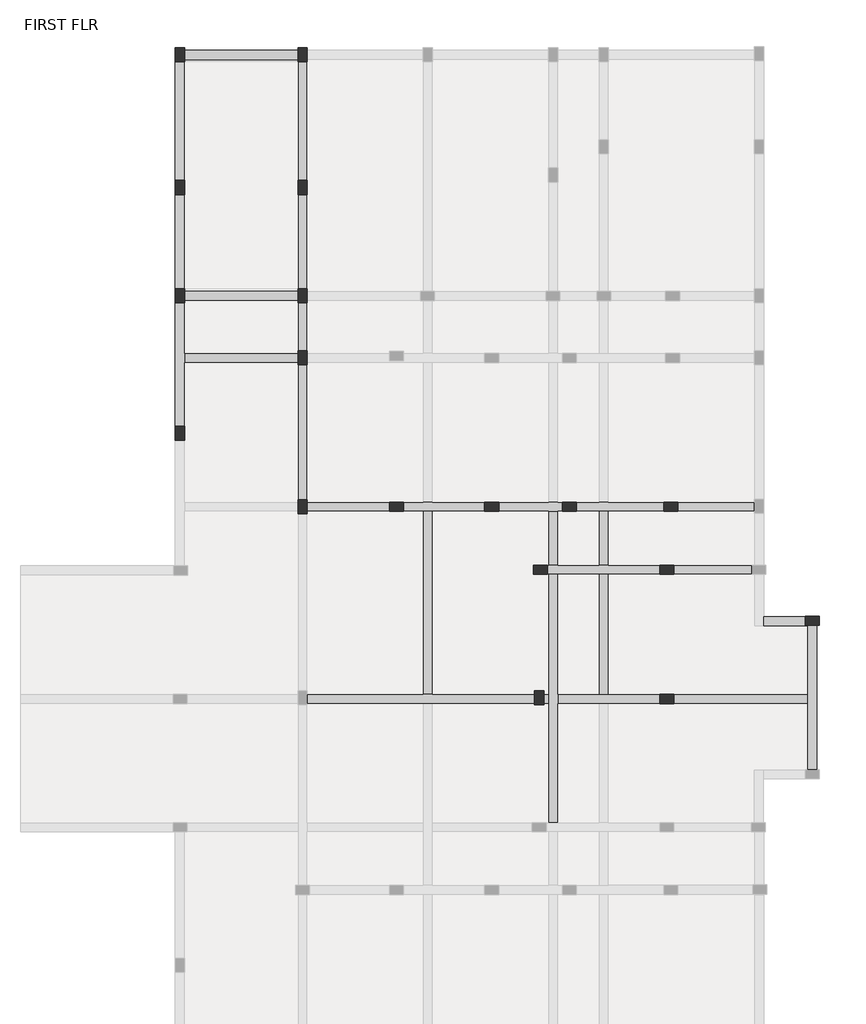
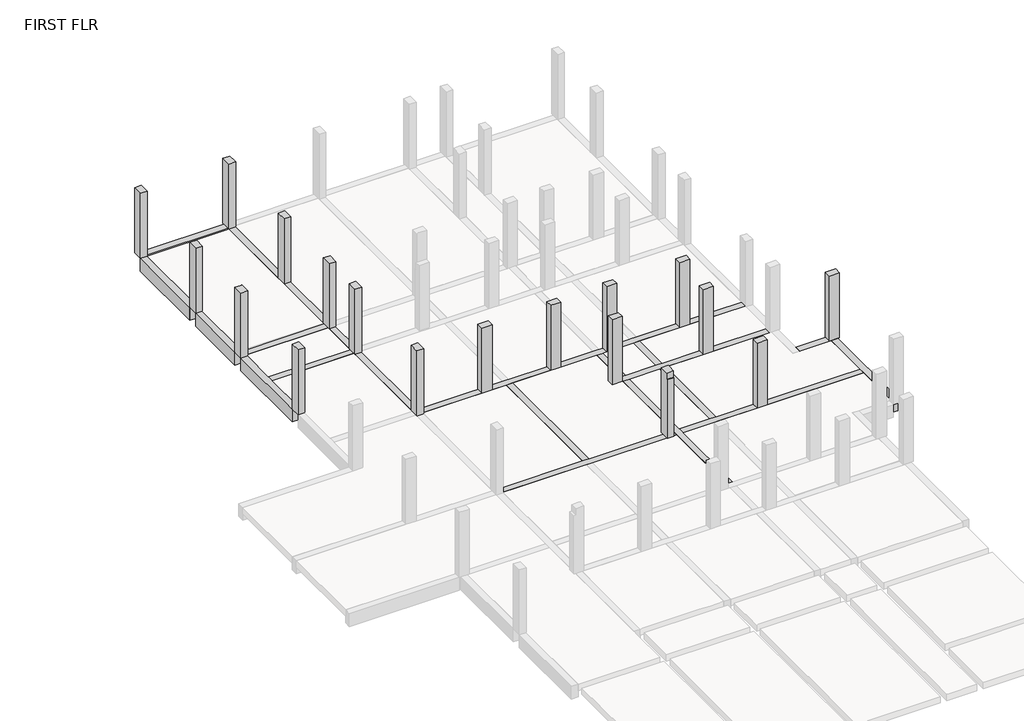
# One storey, part 4 of 5: 28 beams, 18 columns.
"""IFC4 building model written with IfcOpenShell, lengths in millimetres."""

from ifc_helpers import new_model, si_unit, frame, origin, place, context, project, spatial, polyline, outline, extrude, faceted_brep, element, save

model = new_model("IFC4")

# Units and contexts
model_context = context("Model", 3, world=origin())
ifc_project = project(units=[si_unit("LENGTHUNIT", "METRE", prefix="MILLI")], contexts=[model_context])

# Site, building, storey
site = spatial("IfcSite", under=ifc_project)
building = spatial("IfcBuilding", under=site)
storey = spatial("IfcBuildingStorey", under=building, Name="FIRST FLR", Elevation=3000.0)

# Beams
placement = place(None, origin())
element("IfcBeam", 1, ObjectType="M_Concrete-Rectangular Beam : 300 x 600mm", at=placement, inside=storey, context=model_context, shape_type="SweptSolid", body=[
    extrude(outline(polyline([(-1971.7865686, 21837.8349362), (-1971.7865686, 21537.8349362), (-5591.7865686, 21537.8349362), (-5591.7865686, 21837.8349362), (-1971.7865686, 21837.8349362)])), frame((0.0, 0.0, 2400.0), z_axis=(0.0, 0.0, 1.0), x_axis=(1.0, 0.0, 0.0)), (0.0, 0.0, 1.0), 600.0),
])
element("IfcBeam", 2, ObjectType="M_Concrete-Rectangular Beam : 300 x 600mm", at=placement, inside=storey, context=model_context, shape_type="Brep", body=[
    faceted_brep([(-5891.7865686, 21462.8349362, 3000.0), (-5891.7865686, 17662.8349362, 3000.0), (-5888.8105653, 17662.8349362, 3000.0), (-5888.8105653, 17674.7148651, 3000.0), (-5591.7865686, 17674.7148651, 3000.0), (-5591.7865686, 21462.8349362, 3000.0), (-5891.7865686, 21462.8349362, 2400.0), (-5891.7865686, 17662.8349362, 2400.0), (-5591.7865686, 21462.8349362, 2400.0), (-5591.7865686, 17674.7148651, 2400.0), (-5888.8105653, 17674.7148651, 2400.0), (-5888.8105653, 17662.8349362, 2400.0), (-5591.7865686, 17674.7148651, 2700.0), (-5591.7865686, 21462.8349362, 2700.0)], [[[0, 1, 2, 3, 4, 5]], [[1, 0, 6, 7]], [[7, 6, 8, 9, 10, 11]], [[5, 4, 12, 9, 8, 13]], [[8, 6, 0, 5, 13]], [[1, 7, 11, 2]], [[10, 3, 2, 11]], [[3, 10, 9, 12, 4]]]),
])
element("IfcBeam", 3, ObjectType="M_Concrete-Rectangular Beam : 300 x 600mm", at=placement, inside=storey, context=model_context, shape_type="SweptSolid", body=[
    extrude(outline(polyline([(3000.0, -5888.8105653), (2400.0, -5888.8105653), (2400.0, -5588.8105653), (2700.0, -5588.8105653), (2700.0, -5591.7865686), (3000.0, -5591.7865686), (3000.0, -5888.8105653)])), frame((0.0, 14212.5179708, 0.0), z_axis=(0.0, 1.0, 0.0), x_axis=(0.0, 0.0, 1.0)), (0.0, 0.0, 1.0), 3012.1968944),
])
element("IfcBeam", 4, ObjectType="M_Concrete-Rectangular Beam : 300 x 600mm", at=placement, inside=storey, context=model_context, shape_type="Brep", body=[
    faceted_brep([(-5888.8105653, 13762.5179708, 3000.0), (-5888.8105653, 9817.5252033, 3000.0), (-5588.8105653, 9817.5252033, 3000.0), (-5588.8105653, 11857.4075451, 3000.0), (-5588.8105653, 12157.4075451, 3000.0), (-5588.8105653, 13762.5179708, 3000.0), (-5888.8105653, 13762.5179708, 2400.0), (-5888.8105653, 9817.5252033, 2400.0), (-5588.8105653, 13762.5179708, 2400.0), (-5588.8105653, 12157.4075451, 2400.0), (-5588.8105653, 11857.4075451, 2400.0), (-5588.8105653, 9817.5252033, 2400.0), (-5588.8105653, 13762.5179708, 2700.0), (-5588.8105653, 9817.5252033, 2700.0)], [[[0, 1, 2, 3, 4, 5]], [[1, 0, 6, 7]], [[7, 6, 8, 9, 10, 11]], [[11, 10, 9, 8, 12, 5, 4, 3, 2, 13]], [[8, 6, 0, 5, 12]], [[2, 1, 7, 11, 13]]]),
])
element("IfcBeam", 5, ObjectType="M_Concrete-Rectangular Beam : 300 x 600mm", at=placement, inside=storey, context=model_context, shape_type="Brep", body=[
    faceted_brep([(14319.1163908, 3443.0536525, 3000.0), (14619.1163908, 3443.0536525, 3000.0), (14619.1163908, 3443.0536525, 2400.0), (14319.1163908, 3443.0536525, 2400.0), (14319.1163908, 3435.7536525, 3000.0), (14319.1163908, 1251.1713929, 3000.0), (14319.1163908, 951.1713929, 3000.0), (14319.1163908, -1148.8286071, 3000.0), (14619.1163908, -1148.8286071, 3000.0), (14619.1163908, -1148.8286071, 2400.0), (14319.1163908, -1148.8286071, 2400.0), (14319.1163908, 951.1713929, 2400.0), (14319.1163908, 1251.1713929, 2400.0), (14319.1163908, 3435.7536525, 2400.0), (14319.1163908, -1148.8286071, 2700.0)], [[[0, 1, 2, 3]], [[1, 0, 4, 5, 6, 7, 8]], [[2, 1, 8, 9]], [[3, 2, 9, 10, 11, 12, 13]], [[0, 3, 13, 12, 11, 10, 14, 7, 6, 5, 4]], [[7, 14, 10, 9, 8]]]),
])
element("IfcBeam", 6, ObjectType="M_Concrete-Rectangular Beam : 300 x 600mm", at=placement, inside=storey, context=model_context, shape_type="Brep", body=[
    faceted_brep([(12916.8679014, 3735.7536525, 3000.0), (12916.8679014, 3435.7536525, 3000.0), (14319.1163908, 3435.7536525, 3000.0), (14319.1163908, 3443.0536525, 3000.0), (14619.1163908, 3443.0536525, 3000.0), (14619.1163908, 3455.7536525, 3000.0), (14244.1163908, 3455.7536525, 3000.0), (14244.1163908, 3735.7536525, 3000.0), (12916.8679014, 3735.7536525, 2400.0), (14244.1163908, 3735.7536525, 2400.0), (12916.8679014, 3435.7536525, 2400.0), (14244.1163908, 3455.7536525, 2400.0), (14619.1163908, 3455.7536525, 2400.0), (14619.1163908, 3443.0536525, 2400.0), (14319.1163908, 3443.0536525, 2400.0), (14319.1163908, 3435.7536525, 2400.0), (12916.8679014, 3435.7536525, 2700.0), (14319.1163908, 3435.7536525, 2700.0)], [[[0, 1, 2, 3, 4, 5, 6, 7]], [[8, 0, 7, 9]], [[10, 8, 9, 11, 12, 13, 14, 15]], [[2, 1, 16, 10, 15, 17]], [[1, 0, 8, 10, 16]], [[12, 5, 4, 13]], [[7, 6, 11, 9]], [[11, 6, 5, 12]], [[3, 14, 13, 4]], [[14, 3, 2, 17, 15]]]),
])
element("IfcBeam", 7, ObjectType="M_Concrete-Rectangular Beam : 300 x 600mm", at=placement, inside=storey, context=model_context, shape_type="Brep", body=[
    faceted_brep([(-1671.7865686, 21462.8349362, 3000.0), (-1971.7865686, 21462.8349362, 3000.0), (-1971.7865686, 17674.7148651, 3000.0), (-1671.7865686, 17674.7148651, 3000.0), (-1971.7865686, 21462.8349362, 2700.0), (-1971.7865686, 21462.8349362, 2400.0), (-1971.7865686, 17674.7148651, 2400.0), (-1971.7865686, 17674.7148651, 2700.0), (-1671.7865686, 21462.8349362, 2400.0), (-1671.7865686, 17674.7148651, 2400.0), (-1671.7865686, 17674.7148651, 2700.0), (-1671.7865686, 21462.8349362, 2700.0)], [[[0, 1, 2, 3]], [[2, 1, 4, 5, 6, 7]], [[5, 8, 9, 6]], [[0, 3, 10, 9, 8, 11]], [[1, 0, 11, 8, 5, 4]], [[3, 2, 7, 6, 9, 10]]]),
])
element("IfcBeam", 8, ObjectType="M_Concrete-Rectangular Beam : 300 x 600mm", at=placement, inside=storey, context=model_context, shape_type="Brep", body=[
    faceted_brep([(-1671.7865686, 17224.7148651, 3000.0), (-1971.7865686, 17224.7148651, 3000.0), (-1971.7865686, 14212.5179708, 3000.0), (-1671.7865686, 14212.5179708, 3000.0), (-1971.7865686, 17224.7148651, 2700.0), (-1971.7865686, 17224.7148651, 2400.0), (-1971.7865686, 14212.5179708, 2400.0), (-1971.7865686, 14212.5179708, 2700.0), (-1671.7865686, 17224.7148651, 2400.0), (-1671.7865686, 14212.5179708, 2400.0), (-1671.7865686, 14212.5179708, 2700.0), (-1671.7865686, 17224.7148651, 2700.0)], [[[0, 1, 2, 3]], [[2, 1, 4, 5, 6, 7]], [[5, 8, 9, 6]], [[0, 3, 10, 9, 8, 11]], [[1, 0, 11, 8, 5, 4]], [[3, 2, 7, 6, 9, 10]]]),
])
element("IfcBeam", 9, ObjectType="M_Concrete-Rectangular Beam : 300 x 600mm", at=placement, inside=storey, context=model_context, shape_type="Brep", body=[
    faceted_brep([(-1671.7865686, 13762.5179708, 3000.0), (-1971.7865686, 13762.5179708, 3000.0), (-1971.7865686, 12232.4075451, 3000.0), (-1671.7865686, 12232.4075451, 3000.0), (-1971.7865686, 13762.5179708, 2700.0), (-1971.7865686, 13762.5179708, 2400.0), (-1971.7865686, 12232.4075451, 2400.0), (-1971.7865686, 12232.4075451, 2700.0), (-1671.7865686, 13762.5179708, 2400.0), (-1671.7865686, 12232.4075451, 2400.0), (-1671.7865686, 12232.4075451, 2700.0), (-1671.7865686, 13762.5179708, 2700.0)], [[[0, 1, 2, 3]], [[2, 1, 4, 5, 6, 7]], [[5, 8, 9, 6]], [[0, 3, 10, 9, 8, 11]], [[1, 0, 11, 8, 5, 4]], [[3, 2, 7, 6, 9, 10]]]),
])
element("IfcBeam", 10, ObjectType="M_Concrete-Rectangular Beam : 300 x 600mm", at=placement, inside=storey, context=model_context, shape_type="Brep", body=[
    faceted_brep([(-1671.7865686, 11782.4075451, 3000.0), (-1971.7865686, 11782.4075451, 3000.0), (-1971.7865686, 7474.7076276, 3000.0), (-1671.7865686, 7474.7076276, 3000.0), (-1971.7865686, 11782.4075451, 2700.0), (-1971.7865686, 11782.4075451, 2400.0), (-1971.7865686, 7474.7076276, 2400.0), (-1971.7865686, 7474.7076276, 2700.0), (-1671.7865686, 11782.4075451, 2400.0), (-1671.7865686, 7474.7076276, 2400.0), (-1671.7865686, 7474.7076276, 2700.0), (-1671.7865686, 11782.4075451, 2700.0)], [[[0, 1, 2, 3]], [[2, 1, 4, 5, 6, 7]], [[5, 8, 9, 6]], [[0, 3, 10, 9, 8, 11]], [[1, 0, 11, 8, 5, 4]], [[3, 2, 7, 6, 9, 10]]]),
])
element("IfcBeam", 11, ObjectType="M_Concrete-Rectangular Beam : 300 x 600mm", at=placement, inside=storey, context=model_context, shape_type="Brep", body=[
    faceted_brep([(-5588.8105653, 14137.5179708, 3000.0), (-5588.8105653, 13837.5179708, 3000.0), (-1971.7865686, 13837.5179708, 3000.0), (-1971.7865686, 14137.5179708, 3000.0), (-5588.8105653, 13837.5179708, 2700.0), (-5588.8105653, 13837.5179708, 2400.0), (-1971.7865686, 13837.5179708, 2400.0), (-1971.7865686, 13837.5179708, 2700.0), (-5588.8105653, 14137.5179708, 2400.0), (-1971.7865686, 14137.5179708, 2400.0)], [[[0, 1, 2, 3]], [[2, 1, 4, 5, 6, 7]], [[5, 8, 9, 6]], [[8, 0, 3, 9]], [[1, 0, 8, 5, 4]], [[9, 3, 2, 7, 6]]]),
])
element("IfcBeam", 12, ObjectType="M_Concrete-Rectangular Beam : 300 x 600mm", at=placement, inside=storey, context=model_context, shape_type="Brep", body=[
    faceted_brep([(-1971.7865686, 11857.4075451, 3000.0), (-1971.7865686, 12157.4075451, 3000.0), (-5588.8105653, 12157.4075451, 3000.0), (-5588.8105653, 11857.4075451, 3000.0), (-5588.8105653, 11857.4075451, 2700.0), (-5588.8105653, 11857.4075451, 2400.0), (-1971.7865686, 11857.4075451, 2400.0), (-1971.7865686, 11857.4075451, 2700.0), (-1971.7865686, 12157.4075451, 2400.0), (-5588.8105653, 12157.4075451, 2400.0), (-1971.7865686, 12157.4075451, 2700.0), (-5588.8105653, 12157.4075451, 2700.0)], [[[0, 1, 2, 3]], [[0, 3, 4, 5, 6, 7]], [[8, 6, 5, 9]], [[2, 1, 10, 8, 9, 11]], [[1, 0, 7, 6, 8, 10]], [[3, 2, 11, 9, 5, 4]]]),
])
element("IfcBeam", 13, ObjectType="M_Concrete-Rectangular Beam : 300 x 600mm", at=placement, inside=storey, context=model_context, shape_type="Brep", body=[
    faceted_brep([(-1671.7865686, 7399.7076276, 3000.0), (-1671.7865686, 7099.7076276, 3000.0), (949.7296816, 7099.7076276, 3000.0), (949.7296816, 7399.7076276, 3000.0), (-1671.7865686, 7099.7076276, 2700.0), (-1671.7865686, 7099.7076276, 2400.0), (949.7296816, 7099.7076276, 2400.0), (949.7296816, 7099.7076276, 2700.0), (-1671.7865686, 7399.7076276, 2400.0), (949.7296816, 7399.7076276, 2400.0), (949.7296816, 7399.7076276, 2700.0), (-1671.7865686, 7399.7076276, 2700.0)], [[[0, 1, 2, 3]], [[2, 1, 4, 5, 6, 7]], [[5, 8, 9, 6]], [[0, 3, 10, 9, 8, 11]], [[1, 0, 11, 8, 5, 4]], [[3, 2, 7, 6, 9, 10]]]),
])
element("IfcBeam", 14, ObjectType="M_Concrete-Rectangular Beam : 300 x 600mm", at=placement, inside=storey, context=model_context, shape_type="Brep", body=[
    faceted_brep([(1399.7296816, 7399.7076276, 3000.0), (1399.7296816, 7099.7076276, 3000.0), (2024.7296816, 7099.7076276, 3000.0), (2324.7296816, 7099.7076276, 3000.0), (3997.5248054, 7099.7076276, 3000.0), (3997.5248054, 7399.7076276, 3000.0), (2324.7296816, 7399.7076276, 3000.0), (2024.7296816, 7399.7076276, 3000.0), (1399.7296816, 7099.7076276, 2400.0), (2024.7296816, 7099.7076276, 2400.0), (2324.7296816, 7099.7076276, 2400.0), (3997.5248054, 7099.7076276, 2400.0), (3997.5248054, 7099.7076276, 2700.0), (1399.7296816, 7099.7076276, 2700.0), (1399.7296816, 7399.7076276, 2400.0), (2024.7296816, 7399.7076276, 2400.0), (2324.7296816, 7399.7076276, 2400.0), (3997.5248054, 7399.7076276, 2400.0), (1399.7296816, 7399.7076276, 2700.0), (3997.5248054, 7399.7076276, 2700.0)], [[[0, 1, 2, 3, 4, 5, 6, 7]], [[8, 9, 10, 11, 12, 4, 3, 2, 1, 13]], [[8, 14, 15, 16, 17, 11, 10, 9]], [[17, 16, 15, 14, 18, 0, 7, 6, 5, 19]], [[1, 0, 18, 14, 8, 13]], [[5, 4, 12, 11, 17, 19]]]),
])
element("IfcBeam", 15, ObjectType="M_Concrete-Rectangular Beam : 300 x 600mm", at=placement, inside=storey, context=model_context, shape_type="Brep", body=[
    faceted_brep([(4447.5248054, 7399.7076276, 3000.0), (4447.5248054, 7099.7076276, 3000.0), (6032.5248054, 7099.7076276, 3000.0), (6332.5248054, 7099.7076276, 3000.0), (6481.8679014, 7099.7076276, 3000.0), (6481.8679014, 7399.7076276, 3000.0), (6332.5248054, 7399.7076276, 3000.0), (6032.5248054, 7399.7076276, 3000.0), (4447.5248054, 7099.7076276, 2400.0), (6032.5248054, 7099.7076276, 2400.0), (6332.5248054, 7099.7076276, 2400.0), (6481.8679014, 7099.7076276, 2400.0), (6481.8679014, 7099.7076276, 2700.0), (4447.5248054, 7099.7076276, 2700.0), (4447.5248054, 7399.7076276, 2400.0), (6032.5248054, 7399.7076276, 2400.0), (6332.5248054, 7399.7076276, 2400.0), (6481.8679014, 7399.7076276, 2400.0), (4447.5248054, 7399.7076276, 2700.0), (6481.8679014, 7399.7076276, 2700.0)], [[[0, 1, 2, 3, 4, 5, 6, 7]], [[8, 9, 10, 11, 12, 4, 3, 2, 1, 13]], [[8, 14, 15, 16, 17, 11, 10, 9]], [[17, 16, 15, 14, 18, 0, 7, 6, 5, 19]], [[1, 0, 18, 14, 8, 13]], [[5, 4, 12, 11, 17, 19]]]),
])
element("IfcBeam", 16, ObjectType="M_Concrete-Rectangular Beam : 300 x 600mm", at=placement, inside=storey, context=model_context, shape_type="Brep", body=[
    faceted_brep([(6931.8679014, 7399.7076276, 3000.0), (6931.8679014, 7099.7076276, 3000.0), (7656.8679014, 7099.7076276, 3000.0), (7956.8679014, 7099.7076276, 3000.0), (9721.8679014, 7099.7076276, 3000.0), (9721.8679014, 7399.7076276, 3000.0), (7956.8679014, 7399.7076276, 3000.0), (7656.8679014, 7399.7076276, 3000.0), (6931.8679014, 7099.7076276, 2400.0), (7656.8679014, 7099.7076276, 2400.0), (7956.8679014, 7099.7076276, 2400.0), (9721.8679014, 7099.7076276, 2400.0), (9721.8679014, 7099.7076276, 2700.0), (6931.8679014, 7099.7076276, 2700.0), (6931.8679014, 7399.7076276, 2400.0), (7656.8679014, 7399.7076276, 2400.0), (7956.8679014, 7399.7076276, 2400.0), (9721.8679014, 7399.7076276, 2400.0), (6931.8679014, 7399.7076276, 2700.0), (9721.8679014, 7399.7076276, 2700.0)], [[[0, 1, 2, 3, 4, 5, 6, 7]], [[8, 9, 10, 11, 12, 4, 3, 2, 1, 13]], [[8, 14, 15, 16, 17, 11, 10, 9]], [[17, 16, 15, 14, 18, 0, 7, 6, 5, 19]], [[1, 0, 18, 14, 8, 13]], [[5, 4, 12, 11, 17, 19]]]),
])
element("IfcBeam", 17, ObjectType="M_Concrete-Rectangular Beam : 300 x 600mm", at=placement, inside=storey, context=model_context, shape_type="Brep", body=[
    faceted_brep([(6007.5248054, 5387.6057249, 3000.0), (6007.5248054, 5087.6057249, 3000.0), (6032.5248054, 5087.6057249, 3000.0), (6332.5248054, 5087.6057249, 3000.0), (7656.8679014, 5087.6057249, 3000.0), (7956.8679014, 5087.6057249, 3000.0), (9601.8679014, 5087.6057249, 3000.0), (9601.8679014, 5387.6057249, 3000.0), (7956.8679014, 5387.6057249, 3000.0), (7656.8679014, 5387.6057249, 3000.0), (6332.5248054, 5387.6057249, 3000.0), (6032.5248054, 5387.6057249, 3000.0), (6007.5248054, 5087.6057249, 2400.0), (6032.5248054, 5087.6057249, 2400.0), (6332.5248054, 5087.6057249, 2400.0), (7656.8679014, 5087.6057249, 2400.0), (7956.8679014, 5087.6057249, 2400.0), (9601.8679014, 5087.6057249, 2400.0), (9601.8679014, 5087.6057249, 2700.0), (6007.5248054, 5087.6057249, 2700.0), (6007.5248054, 5387.6057249, 2400.0), (6032.5248054, 5387.6057249, 2400.0), (6332.5248054, 5387.6057249, 2400.0), (7656.8679014, 5387.6057249, 2400.0), (7956.8679014, 5387.6057249, 2400.0), (9601.8679014, 5387.6057249, 2400.0), (6007.5248054, 5387.6057249, 2700.0), (9601.8679014, 5387.6057249, 2700.0)], [[[0, 1, 2, 3, 4, 5, 6, 7, 8, 9, 10, 11]], [[12, 13, 14, 15, 16, 17, 18, 6, 5, 4, 3, 2, 1, 19]], [[12, 20, 21, 22, 23, 24, 25, 17, 16, 15, 14, 13]], [[25, 24, 23, 22, 21, 20, 26, 0, 11, 10, 9, 8, 7, 27]], [[1, 0, 26, 20, 12, 19]], [[7, 6, 18, 17, 25, 27]]]),
])
element("IfcBeam", 18, ObjectType="M_Concrete-Rectangular Beam : 300 x 600mm", at=placement, inside=storey, context=model_context, shape_type="Brep", body=[
    faceted_brep([(10051.8679014, 5387.6057249, 3000.0), (10051.8679014, 5087.6057249, 3000.0), (12541.8679014, 5087.6057249, 3000.0), (12541.8679014, 5387.6057249, 3000.0), (10051.8679014, 5087.6057249, 2700.0), (10051.8679014, 5087.6057249, 2400.0), (12541.8679014, 5087.6057249, 2400.0), (12541.8679014, 5087.6057249, 2700.0), (10051.8679014, 5387.6057249, 2400.0), (12541.8679014, 5387.6057249, 2400.0), (12541.8679014, 5387.6057249, 2700.0), (10051.8679014, 5387.6057249, 2700.0)], [[[0, 1, 2, 3]], [[2, 1, 4, 5, 6, 7]], [[5, 8, 9, 6]], [[0, 3, 10, 9, 8, 11]], [[1, 0, 11, 8, 5, 4]], [[3, 2, 7, 6, 9, 10]]]),
])
element("IfcBeam", 19, ObjectType="M_Concrete-Rectangular Beam : 300 x 600mm", at=placement, inside=storey, context=model_context, shape_type="Brep", body=[
    faceted_brep([(10051.8679014, 1251.1713929, 3000.0), (10051.8679014, 951.1713929, 3000.0), (14319.1163908, 951.1713929, 3000.0), (14319.1163908, 1251.1713929, 3000.0), (10051.8679014, 951.1713929, 2700.0), (10051.8679014, 951.1713929, 2400.0), (14319.1163908, 951.1713929, 2400.0), (14319.1163908, 951.1713929, 2700.0), (10051.8679014, 1251.1713929, 2400.0), (14319.1163908, 1251.1713929, 2400.0), (14319.1163908, 1251.1713929, 2700.0), (10051.8679014, 1251.1713929, 2700.0)], [[[0, 1, 2, 3]], [[2, 1, 4, 5, 6, 7]], [[5, 8, 9, 6]], [[0, 3, 10, 9, 8, 11]], [[1, 0, 11, 8, 5, 4]], [[3, 2, 7, 6, 9, 10]]]),
])
element("IfcBeam", 20, ObjectType="M_Concrete-Rectangular Beam : 300 x 600mm", at=placement, inside=storey, context=model_context, shape_type="Brep", body=[
    faceted_brep([(6032.5248054, 951.1713929, 3000.0), (6032.5248054, 1251.1713929, 3000.0), (5892.5248054, 1251.1713929, 3000.0), (5892.5248054, 951.1713929, 3000.0), (5892.5248054, 951.1713929, 2700.0), (5892.5248054, 951.1713929, 2400.0), (6032.5248054, 951.1713929, 2400.0), (6032.5248054, 951.1713929, 2700.0), (6032.5248054, 1251.1713929, 2400.0), (5892.5248054, 1251.1713929, 2400.0), (6032.5248054, 1251.1713929, 2700.0), (5892.5248054, 1251.1713929, 2700.0)], [[[0, 1, 2, 3]], [[0, 3, 4, 5, 6, 7]], [[8, 6, 5, 9]], [[2, 1, 10, 8, 9, 11]], [[1, 0, 7, 6, 8, 10]], [[3, 2, 11, 9, 5, 4]]]),
    faceted_brep([(-1671.7865686, 951.1713929, 3000.0), (-1671.7865686, 1251.1713929, 3000.0), (-1671.7865686, 1251.1713929, 2700.0), (-1671.7865686, 1251.1713929, 2400.0), (-1671.7865686, 951.1713929, 2400.0), (-1671.7865686, 951.1713929, 2700.0), (5592.5248054, 1251.1713929, 3000.0), (5592.5248054, 951.1713929, 3000.0), (5592.5248054, 951.1713929, 2700.0), (5592.5248054, 951.1713929, 2400.0), (5592.5248054, 1251.1713929, 2400.0), (5592.5248054, 1251.1713929, 2700.0), (2024.7296816, 951.1713929, 3000.0), (2324.7296816, 951.1713929, 3000.0), (2324.7296816, 1251.1713929, 3000.0), (2024.7296816, 1251.1713929, 3000.0), (2024.7296816, 951.1713929, 2400.0), (2324.7296816, 951.1713929, 2400.0), (2024.7296816, 1251.1713929, 2400.0), (2324.7296816, 1251.1713929, 2400.0)], [[[0, 1, 2, 3, 4, 5]], [[6, 7, 8, 9, 10, 11]], [[1, 0, 12, 13, 7, 6, 14, 15]], [[4, 16, 17, 9, 8, 7, 13, 12, 0, 5]], [[4, 3, 18, 19, 10, 9, 17, 16]], [[10, 19, 18, 3, 2, 1, 15, 14, 6, 11]]]),
])
element("IfcBeam", 21, ObjectType="M_Concrete-Rectangular Beam : 300 x 600mm", at=placement, inside=storey, context=model_context, shape_type="Brep", body=[
    faceted_brep([(2324.7296816, 7099.7076276, 3000.0), (2024.7296816, 7099.7076276, 3000.0), (2024.7296816, 1251.1713929, 3000.0), (2324.7296816, 1251.1713929, 3000.0), (2024.7296816, 7099.7076276, 2700.0), (2024.7296816, 7099.7076276, 2400.0), (2024.7296816, 1251.1713929, 2400.0), (2024.7296816, 1251.1713929, 2700.0), (2324.7296816, 7099.7076276, 2400.0), (2324.7296816, 5387.6057249, 2400.0), (2324.7296816, 5087.6057249, 2400.0), (2324.7296816, 1251.1713929, 2400.0), (2324.7296816, 1251.1713929, 2700.0), (2324.7296816, 7099.7076276, 2700.0)], [[[0, 1, 2, 3]], [[2, 1, 4, 5, 6, 7]], [[5, 8, 9, 10, 11, 6]], [[0, 3, 12, 11, 10, 9, 8, 13]], [[1, 0, 13, 8, 5, 4]], [[3, 2, 7, 6, 11, 12]]]),
])
element("IfcBeam", 22, ObjectType="M_Concrete-Rectangular Beam : 300 x 600mm", at=placement, inside=storey, context=model_context, shape_type="Brep", body=[
    faceted_brep([(6332.5248054, 7099.7076276, 3000.0), (6032.5248054, 7099.7076276, 3000.0), (6032.5248054, 5387.6057249, 3000.0), (6332.5248054, 5387.6057249, 3000.0), (6032.5248054, 7099.7076276, 2700.0), (6032.5248054, 7099.7076276, 2400.0), (6032.5248054, 5387.6057249, 2400.0), (6032.5248054, 5387.6057249, 2700.0), (6332.5248054, 7099.7076276, 2400.0), (6332.5248054, 5387.6057249, 2400.0), (6332.5248054, 5387.6057249, 2700.0), (6332.5248054, 7099.7076276, 2700.0)], [[[0, 1, 2, 3]], [[2, 1, 4, 5, 6, 7]], [[5, 8, 9, 6]], [[0, 3, 10, 9, 8, 11]], [[1, 0, 11, 8, 5, 4]], [[3, 2, 7, 6, 9, 10]]]),
])
element("IfcBeam", 23, ObjectType="M_Concrete-Rectangular Beam : 300 x 600mm", at=placement, inside=storey, context=model_context, shape_type="Brep", body=[
    faceted_brep([(7956.8679014, 7099.7076276, 3000.0), (7656.8679014, 7099.7076276, 3000.0), (7656.8679014, 5387.6057249, 3000.0), (7956.8679014, 5387.6057249, 3000.0), (7656.8679014, 7099.7076276, 2700.0), (7656.8679014, 7099.7076276, 2400.0), (7656.8679014, 5387.6057249, 2400.0), (7656.8679014, 5387.6057249, 2700.0), (7956.8679014, 7099.7076276, 2400.0), (7956.8679014, 5387.6057249, 2400.0), (7956.8679014, 5387.6057249, 2700.0), (7956.8679014, 7099.7076276, 2700.0)], [[[0, 1, 2, 3]], [[2, 1, 4, 5, 6, 7]], [[5, 8, 9, 6]], [[0, 3, 10, 9, 8, 11]], [[1, 0, 11, 8, 5, 4]], [[3, 2, 7, 6, 9, 10]]]),
])
element("IfcBeam", 24, ObjectType="M_Concrete-Rectangular Beam : 300 x 600mm", at=placement, inside=storey, context=model_context, shape_type="Brep", body=[
    faceted_brep([(6332.5248054, 5087.6057249, 3000.0), (6032.5248054, 5087.6057249, 3000.0), (6032.5248054, 1251.1713929, 3000.0), (6032.5248054, 951.1713929, 3000.0), (6032.5248054, -2839.4535766, 3000.0), (6332.5248054, -2839.4535766, 3000.0), (6332.5248054, 951.1713929, 3000.0), (6332.5248054, 1251.1713929, 3000.0), (6032.5248054, 5087.6057249, 2400.0), (6032.5248054, 1251.1713929, 2400.0), (6032.5248054, 951.1713929, 2400.0), (6032.5248054, -2839.4535766, 2400.0), (6032.5248054, -2839.4535766, 2700.0), (6032.5248054, 5087.6057249, 2700.0), (6332.5248054, 5087.6057249, 2400.0), (6332.5248054, 1251.1713929, 2400.0), (6332.5248054, 951.1713929, 2400.0), (6332.5248054, -2839.4535766, 2400.0), (6332.5248054, 5087.6057249, 2700.0), (6332.5248054, -2839.4535766, 2700.0)], [[[0, 1, 2, 3, 4, 5, 6, 7]], [[8, 9, 10, 11, 12, 4, 3, 2, 1, 13]], [[8, 14, 15, 16, 17, 11, 10, 9]], [[17, 16, 15, 14, 18, 0, 7, 6, 5, 19]], [[1, 0, 18, 14, 8, 13]], [[5, 4, 12, 11, 17, 19]]]),
])
element("IfcBeam", 25, ObjectType="M_Concrete-Rectangular Beam : 300 x 600mm", at=placement, inside=storey, context=model_context, shape_type="Brep", body=[
    faceted_brep([(7956.8679014, 5087.6057249, 3000.0), (7656.8679014, 5087.6057249, 3000.0), (7656.8679014, 1251.1713929, 3000.0), (7956.8679014, 1251.1713929, 3000.0), (7656.8679014, 5087.6057249, 2700.0), (7656.8679014, 5087.6057249, 2400.0), (7656.8679014, 1251.1713929, 2400.0), (7656.8679014, 1251.1713929, 2700.0), (7956.8679014, 5087.6057249, 2400.0), (7956.8679014, 1251.1713929, 2400.0), (7956.8679014, 1251.1713929, 2700.0), (7956.8679014, 5087.6057249, 2700.0)], [[[0, 1, 2, 3]], [[2, 1, 4, 5, 6, 7]], [[5, 8, 9, 6]], [[0, 3, 10, 9, 8, 11]], [[1, 0, 11, 8, 5, 4]], [[3, 2, 7, 6, 9, 10]]]),
])
element("IfcBeam", 26, ObjectType="M_Concrete-Rectangular Beam : 300 x 600mm", at=placement, inside=storey, context=model_context, shape_type="Brep", body=[
    faceted_brep([(9601.8679014, 951.1713929, 3000.0), (9601.8679014, 1251.1713929, 3000.0), (7956.8679014, 1251.1713929, 3000.0), (7656.8679014, 1251.1713929, 3000.0), (6332.5248054, 1251.1713929, 3000.0), (6332.5248054, 951.1713929, 3000.0), (7656.8679014, 951.1713929, 3000.0), (7956.8679014, 951.1713929, 3000.0), (6332.5248054, 951.1713929, 2400.0), (7656.8679014, 951.1713929, 2400.0), (7956.8679014, 951.1713929, 2400.0), (9601.8679014, 951.1713929, 2400.0), (9601.8679014, 951.1713929, 2700.0), (6332.5248054, 951.1713929, 2700.0), (9601.8679014, 1251.1713929, 2400.0), (6332.5248054, 1251.1713929, 2400.0), (7656.8679014, 1251.1713929, 2400.0), (7956.8679014, 1251.1713929, 2400.0), (6332.5248054, 1251.1713929, 2700.0), (9601.8679014, 1251.1713929, 2700.0)], [[[0, 1, 2, 3, 4, 5, 6, 7]], [[8, 9, 10, 11, 12, 0, 7, 6, 5, 13]], [[14, 11, 10, 9, 8, 15, 16, 17]], [[14, 17, 16, 15, 18, 4, 3, 2, 1, 19]], [[1, 0, 12, 11, 14, 19]], [[5, 4, 18, 15, 8, 13]]]),
])
element("IfcBeam", 27, ObjectType="M_Concrete-Rectangular Beam : 300 x 600mm", at=placement, inside=storey, context=model_context, shape_type="Brep", body=[
    faceted_brep([(10171.8679014, 7399.7076276, 3000.0), (10171.8679014, 7099.7076276, 3000.0), (12616.8679014, 7099.7076276, 3000.0), (12616.8679014, 7399.7076276, 3000.0), (10171.8679014, 7099.7076276, 2700.0), (10171.8679014, 7099.7076276, 2400.0), (12616.8679014, 7099.7076276, 2400.0), (12616.8679014, 7099.7076276, 2700.0), (10171.8679014, 7399.7076276, 2400.0), (12616.8679014, 7399.7076276, 2400.0), (12616.8679014, 7399.7076276, 2700.0), (10171.8679014, 7399.7076276, 2700.0)], [[[0, 1, 2, 3]], [[2, 1, 4, 5, 6, 7]], [[5, 8, 9, 6]], [[0, 3, 10, 9, 8, 11]], [[8, 5, 4, 1, 0, 11]], [[3, 2, 7, 6, 9, 10]]]),
])
element("IfcBeam", 28, ObjectType="M_Concrete-Rectangular Beam : 300 x 600mm", at=placement, inside=storey, context=model_context, shape_type="SweptSolid", body=[
    extrude(outline(polyline([(5557.5248054, 5387.6057249), (5557.5248054, 5087.6057249), (2324.7296816, 5087.6057249), (2324.7296816, 5387.6057249), (5557.5248054, 5387.6057249)])), frame((0.0, 0.0, 2400.0), z_axis=(0.0, 0.0, 1.0), x_axis=(1.0, 0.0, 0.0)), (0.0, 0.0, 1.0), 300.0),
])

# Columns
element("IfcColumn", 29, ObjectType="M_Concrete-Rectangular-Column : 300 x 450mm", at=placement, inside=storey, context=model_context, shape_type="SweptSolid", body=[
    extrude(outline(polyline([(-5591.7865686, 21912.8349362), (-5591.7865686, 21462.8349362), (-5891.7865686, 21462.8349362), (-5891.7865686, 21912.8349362), (-5591.7865686, 21912.8349362)])), frame((0.0, 0.0, 3000.0), z_axis=(0.0, 0.0, 1.0), x_axis=(1.0, 0.0, 0.0)), (0.0, 0.0, 1.0), 3048.0),
])
element("IfcColumn", 30, ObjectType="M_Concrete-Rectangular-Column : 300 x 450mm", at=placement, inside=storey, context=model_context, shape_type="Brep", body=[
    faceted_brep([(-1671.7865686, 21912.8349362, 3000.0), (-1671.7865686, 21462.8349362, 3000.0), (-1971.7865686, 21462.8349362, 3000.0), (-1971.7865686, 21912.8349362, 3000.0), (-1671.7865686, 21912.8349362, 6048.0), (-1671.7865686, 21537.8349362, 6048.0), (-1671.7865686, 21462.8349362, 6048.0), (-1671.7865686, 21462.8349362, 5748.0), (-1971.7865686, 21462.8349362, 6048.0), (-1971.7865686, 21462.8349362, 5748.0), (-1971.7865686, 21912.8349362, 6048.0)], [[[0, 1, 2, 3]], [[1, 0, 4, 5, 6, 7]], [[2, 1, 7, 6, 8, 9]], [[3, 2, 9, 8, 10]], [[0, 3, 10, 4]], [[8, 6, 5, 4, 10]]]),
])
element("IfcColumn", 31, ObjectType="M_Concrete-Rectangular-Column : 300 x 450mm", at=placement, inside=storey, context=model_context, shape_type="Brep", body=[
    faceted_brep([(-1671.7865686, 17674.7148651, 3000.0), (-1671.7865686, 17224.7148651, 3000.0), (-1971.7865686, 17224.7148651, 3000.0), (-1971.7865686, 17674.7148651, 3000.0), (-1671.7865686, 17674.7148651, 5748.0), (-1671.7865686, 17674.7148651, 6048.0), (-1671.7865686, 17224.7148651, 6048.0), (-1671.7865686, 17224.7148651, 5748.0), (-1971.7865686, 17224.7148651, 6048.0), (-1971.7865686, 17224.7148651, 5748.0), (-1971.7865686, 17674.7148651, 6048.0), (-1971.7865686, 17674.7148651, 5748.0)], [[[0, 1, 2, 3]], [[1, 0, 4, 5, 6, 7]], [[2, 1, 7, 6, 8, 9]], [[3, 2, 9, 8, 10, 11]], [[0, 3, 11, 10, 5, 4]], [[6, 5, 10, 8]]]),
])
element("IfcColumn", 32, ObjectType="M_Concrete-Rectangular-Column : 300 x 450mm", at=placement, inside=storey, context=model_context, shape_type="SweptSolid", body=[
    extrude(outline(polyline([(3000.0, -5888.8105653), (3000.0, -5588.8105653), (5748.0, -5588.8105653), (5748.0, -5591.7865686), (6048.0, -5591.7865686), (6048.0, -5888.8105653), (3000.0, -5888.8105653)])), frame((0.0, 17224.7148651, 0.0), z_axis=(0.0, 1.0, 0.0), x_axis=(0.0, 0.0, 1.0)), (0.0, 0.0, 1.0), 450.0),
])
element("IfcColumn", 33, ObjectType="M_Concrete-Rectangular-Column : 300 x 450mm", at=placement, inside=storey, context=model_context, shape_type="Brep", body=[
    faceted_brep([(-5588.8105653, 14212.5179708, 3000.0), (-5588.8105653, 13762.5179708, 3000.0), (-5888.8105653, 13762.5179708, 3000.0), (-5888.8105653, 14212.5179708, 3000.0), (-5588.8105653, 14212.5179708, 5748.0), (-5588.8105653, 14212.5179708, 6048.0), (-5588.8105653, 13837.5179708, 6048.0), (-5588.8105653, 13762.5179708, 6048.0), (-5588.8105653, 13762.5179708, 5748.0), (-5888.8105653, 13762.5179708, 6048.0), (-5888.8105653, 14212.5179708, 6048.0), (-5591.7865686, 14212.5179708, 6048.0)], [[[0, 1, 2, 3]], [[1, 0, 4, 5, 6, 7, 8]], [[2, 1, 8, 7, 9]], [[3, 2, 9, 10]], [[0, 3, 10, 11, 5, 4]], [[9, 7, 6, 5, 11, 10]]]),
])
element("IfcColumn", 34, ObjectType="M_Concrete-Rectangular-Column : 300 x 450mm", at=placement, inside=storey, context=model_context, shape_type="Brep", body=[
    faceted_brep([(-1671.7865686, 14212.5179708, 3000.0), (-1671.7865686, 13762.5179708, 3000.0), (-1971.7865686, 13762.5179708, 3000.0), (-1971.7865686, 14212.5179708, 3000.0), (-1671.7865686, 14212.5179708, 5748.0), (-1671.7865686, 14212.5179708, 6048.0), (-1671.7865686, 14137.5179708, 6048.0), (-1671.7865686, 13837.5179708, 6048.0), (-1671.7865686, 13762.5179708, 6048.0), (-1671.7865686, 13762.5179708, 5748.0), (-1971.7865686, 13762.5179708, 6048.0), (-1971.7865686, 13762.5179708, 5748.0), (-1971.7865686, 13837.5179708, 6048.0), (-1971.7865686, 14212.5179708, 6048.0), (-1971.7865686, 14212.5179708, 5748.0)], [[[0, 1, 2, 3]], [[1, 0, 4, 5, 6, 7, 8, 9]], [[2, 1, 9, 8, 10, 11]], [[3, 2, 11, 10, 12, 13, 14]], [[0, 3, 14, 13, 5, 4]], [[10, 8, 7, 6, 5, 13, 12]]]),
])
element("IfcColumn", 35, ObjectType="M_Concrete-Rectangular-Column : 300 x 450mm", at=placement, inside=storey, context=model_context, shape_type="Brep", body=[
    faceted_brep([(-1971.7865686, 11782.4075451, 3000.0), (-1971.7865686, 12232.4075451, 3000.0), (-1671.7865686, 12232.4075451, 3000.0), (-1671.7865686, 11782.4075451, 3000.0), (-1971.7865686, 11782.4075451, 5748.0), (-1971.7865686, 11782.4075451, 6048.0), (-1971.7865686, 11857.4075451, 6048.0), (-1971.7865686, 12157.4075451, 6048.0), (-1971.7865686, 12232.4075451, 6048.0), (-1971.7865686, 12232.4075451, 5748.0), (-1671.7865686, 12232.4075451, 6048.0), (-1671.7865686, 12232.4075451, 5748.0), (-1671.7865686, 12157.4075451, 6048.0), (-1671.7865686, 11857.4075451, 6048.0), (-1671.7865686, 11782.4075451, 6048.0), (-1671.7865686, 11782.4075451, 5748.0)], [[[0, 1, 2, 3]], [[1, 0, 4, 5, 6, 7, 8, 9]], [[2, 1, 9, 8, 10, 11]], [[3, 2, 11, 10, 12, 13, 14, 15]], [[0, 3, 15, 14, 5, 4]], [[10, 8, 7, 6, 5, 14, 13, 12]]]),
])
element("IfcColumn", 36, ObjectType="M_Concrete-Rectangular-Column : 300 x 450mm", at=placement, inside=storey, context=model_context, shape_type="Brep", body=[
    faceted_brep([(-5888.8105653, 9367.5252033, 3000.0), (-5888.8105653, 9817.5252033, 3000.0), (-5588.8105653, 9817.5252033, 3000.0), (-5588.8105653, 9367.5252033, 3000.0), (-5888.8105653, 9367.5252033, 6048.0), (-5888.8105653, 9817.5252033, 6048.0), (-5588.8105653, 9817.5252033, 6048.0), (-5588.8105653, 9817.5252033, 5748.0), (-5588.8105653, 9367.5252033, 6048.0), (-5588.8105653, 9367.5252033, 5748.0)], [[[0, 1, 2, 3]], [[1, 0, 4, 5]], [[2, 1, 5, 6, 7]], [[3, 2, 7, 6, 8, 9]], [[0, 3, 9, 8, 4]], [[5, 4, 8, 6]]]),
])
element("IfcColumn", 37, ObjectType="M_Concrete-Rectangular-Column : 300 x 450mm", at=placement, inside=storey, context=model_context, shape_type="Brep", body=[
    faceted_brep([(-1971.7865686, 7024.7076276, 3000.0), (-1971.7865686, 7474.7076276, 3000.0), (-1671.7865686, 7474.7076276, 3000.0), (-1671.7865686, 7024.7076276, 3000.0), (-1971.7865686, 7024.7076276, 5748.0), (-1971.7865686, 7024.7076276, 6048.0), (-1971.7865686, 7099.7076276, 6048.0), (-1971.7865686, 7399.7076276, 6048.0), (-1971.7865686, 7474.7076276, 6048.0), (-1971.7865686, 7474.7076276, 5748.0), (-1671.7865686, 7474.7076276, 6048.0), (-1671.7865686, 7474.7076276, 5748.0), (-1671.7865686, 7399.7076276, 6048.0), (-1671.7865686, 7099.7076276, 6048.0), (-1671.7865686, 7024.7076276, 6048.0), (-1671.7865686, 7024.7076276, 5748.0)], [[[0, 1, 2, 3]], [[1, 0, 4, 5, 6, 7, 8, 9]], [[2, 1, 9, 8, 10, 11]], [[3, 2, 11, 10, 12, 13, 14, 15]], [[0, 3, 15, 14, 5, 4]], [[10, 8, 7, 6, 5, 14, 13, 12]]]),
])
element("IfcColumn", 38, ObjectType="M_Concrete-Rectangular-Column : 300 x 450mm", at=placement, inside=storey, context=model_context, shape_type="Brep", body=[
    faceted_brep([(1399.7296816, 7099.7076276, 3000.0), (949.7296816, 7099.7076276, 3000.0), (949.7296816, 7399.7076276, 3000.0), (1399.7296816, 7399.7076276, 3000.0), (1399.7296816, 7099.7076276, 5748.0), (1399.7296816, 7099.7076276, 6048.0), (949.7296816, 7099.7076276, 6048.0), (949.7296816, 7099.7076276, 5748.0), (949.7296816, 7399.7076276, 6048.0), (949.7296816, 7399.7076276, 5748.0), (1399.7296816, 7399.7076276, 6048.0), (1399.7296816, 7399.7076276, 5748.0)], [[[0, 1, 2, 3]], [[1, 0, 4, 5, 6, 7]], [[2, 1, 7, 6, 8, 9]], [[3, 2, 9, 8, 10, 11]], [[0, 3, 11, 10, 5, 4]], [[6, 5, 10, 8]]]),
])
element("IfcColumn", 39, ObjectType="M_Concrete-Rectangular-Column : 300 x 450mm", at=placement, inside=storey, context=model_context, shape_type="Brep", body=[
    faceted_brep([(4447.5248054, 7099.7076276, 3000.0), (3997.5248054, 7099.7076276, 3000.0), (3997.5248054, 7399.7076276, 3000.0), (4447.5248054, 7399.7076276, 3000.0), (4447.5248054, 7099.7076276, 5748.0), (4447.5248054, 7099.7076276, 6048.0), (3997.5248054, 7099.7076276, 6048.0), (3997.5248054, 7099.7076276, 5748.0), (3997.5248054, 7399.7076276, 6048.0), (3997.5248054, 7399.7076276, 5748.0), (4447.5248054, 7399.7076276, 6048.0), (4447.5248054, 7399.7076276, 5748.0)], [[[0, 1, 2, 3]], [[1, 0, 4, 5, 6, 7]], [[2, 1, 7, 6, 8, 9]], [[3, 2, 9, 8, 10, 11]], [[0, 3, 11, 10, 5, 4]], [[6, 5, 10, 8]]]),
])
element("IfcColumn", 40, ObjectType="M_Concrete-Rectangular-Column : 300 x 450mm", at=placement, inside=storey, context=model_context, shape_type="Brep", body=[
    faceted_brep([(6931.8679014, 7099.7076276, 3000.0), (6481.8679014, 7099.7076276, 3000.0), (6481.8679014, 7399.7076276, 3000.0), (6931.8679014, 7399.7076276, 3000.0), (6931.8679014, 7099.7076276, 5748.0), (6931.8679014, 7099.7076276, 6048.0), (6481.8679014, 7099.7076276, 6048.0), (6481.8679014, 7099.7076276, 5748.0), (6481.8679014, 7399.7076276, 6048.0), (6481.8679014, 7399.7076276, 5748.0), (6931.8679014, 7399.7076276, 6048.0), (6931.8679014, 7399.7076276, 5748.0)], [[[0, 1, 2, 3]], [[1, 0, 4, 5, 6, 7]], [[2, 1, 7, 6, 8, 9]], [[3, 2, 9, 8, 10, 11]], [[0, 3, 11, 10, 5, 4]], [[6, 5, 10, 8]]]),
])
element("IfcColumn", 41, ObjectType="M_Concrete-Rectangular-Column : 300 x 450mm", at=placement, inside=storey, context=model_context, shape_type="Brep", body=[
    faceted_brep([(10171.8679014, 7099.7076276, 3000.0), (9721.8679014, 7099.7076276, 3000.0), (9721.8679014, 7399.7076276, 3000.0), (10171.8679014, 7399.7076276, 3000.0), (10171.8679014, 7099.7076276, 5748.0), (10171.8679014, 7099.7076276, 6048.0), (9721.8679014, 7099.7076276, 6048.0), (9721.8679014, 7099.7076276, 5748.0), (9721.8679014, 7399.7076276, 6048.0), (9721.8679014, 7399.7076276, 5748.0), (10171.8679014, 7399.7076276, 6048.0), (10171.8679014, 7399.7076276, 5748.0)], [[[0, 1, 2, 3]], [[1, 0, 4, 5, 6, 7]], [[2, 1, 7, 6, 8, 9]], [[3, 2, 9, 8, 10, 11]], [[0, 3, 11, 10, 5, 4]], [[6, 5, 10, 8]]]),
])
element("IfcColumn", 42, ObjectType="M_Concrete-Rectangular-Column : 300 x 450mm", at=placement, inside=storey, context=model_context, shape_type="Brep", body=[
    faceted_brep([(5557.5248054, 5387.6057249, 3000.0), (6007.5248054, 5387.6057249, 3000.0), (6007.5248054, 5087.6057249, 3000.0), (5557.5248054, 5087.6057249, 3000.0), (5557.5248054, 5387.6057249, 5748.0), (5557.5248054, 5387.6057249, 6048.0), (6007.5248054, 5387.6057249, 6048.0), (6007.5248054, 5387.6057249, 5748.0), (6007.5248054, 5087.6057249, 6048.0), (6007.5248054, 5087.6057249, 5748.0), (5557.5248054, 5087.6057249, 6048.0), (5557.5248054, 5087.6057249, 5748.0)], [[[0, 1, 2, 3]], [[1, 0, 4, 5, 6, 7]], [[2, 1, 7, 6, 8, 9]], [[3, 2, 9, 8, 10, 11]], [[0, 3, 11, 10, 5, 4]], [[6, 5, 10, 8]]]),
])
element("IfcColumn", 43, ObjectType="M_Concrete-Rectangular-Column : 300 x 450mm", at=placement, inside=storey, context=model_context, shape_type="Brep", body=[
    faceted_brep([(9601.8679014, 5387.6057249, 3000.0), (10051.8679014, 5387.6057249, 3000.0), (10051.8679014, 5087.6057249, 3000.0), (9601.8679014, 5087.6057249, 3000.0), (9601.8679014, 5387.6057249, 5748.0), (9601.8679014, 5387.6057249, 6048.0), (10051.8679014, 5387.6057249, 6048.0), (10051.8679014, 5387.6057249, 5748.0), (10051.8679014, 5087.6057249, 6048.0), (10051.8679014, 5087.6057249, 5748.0), (9601.8679014, 5087.6057249, 6048.0), (9601.8679014, 5087.6057249, 5748.0)], [[[0, 1, 2, 3]], [[1, 0, 4, 5, 6, 7]], [[2, 1, 7, 6, 8, 9]], [[3, 2, 9, 8, 10, 11]], [[0, 3, 11, 10, 5, 4]], [[6, 5, 10, 8]]]),
])
element("IfcColumn", 44, ObjectType="M_Concrete-Rectangular-Column : 300 x 450mm", at=placement, inside=storey, context=model_context, shape_type="Brep", body=[
    faceted_brep([(5892.5248054, 1366.1713929, 3000.0), (5892.5248054, 916.1713929, 3000.0), (5592.5248054, 916.1713929, 3000.0), (5592.5248054, 1366.1713929, 3000.0), (5892.5248054, 1366.1713929, 5748.0), (5892.5248054, 1366.1713929, 6048.0), (5892.5248054, 1251.1713929, 6048.0), (5892.5248054, 951.1713929, 6048.0), (5892.5248054, 951.1713929, 5748.0), (5892.5248054, 916.1713929, 5748.0), (5592.5248054, 916.1713929, 5748.0), (5592.5248054, 951.1713929, 5748.0), (5592.5248054, 951.1713929, 6048.0), (5592.5248054, 1251.1713929, 6048.0), (5592.5248054, 1366.1713929, 6048.0), (5592.5248054, 1366.1713929, 5748.0)], [[[0, 1, 2, 3]], [[1, 0, 4, 5, 6, 7, 8, 9]], [[2, 1, 9, 10]], [[3, 2, 10, 11, 12, 13, 14, 15]], [[0, 3, 15, 14, 5, 4]], [[5, 14, 13, 12, 7, 6]], [[8, 11, 10, 9]], [[11, 8, 7, 12]]]),
])
element("IfcColumn", 45, ObjectType="M_Concrete-Rectangular-Column : 300 x 450mm", at=placement, inside=storey, context=model_context, shape_type="Brep", body=[
    faceted_brep([(9601.8679014, 1251.1713929, 3000.0), (10051.8679014, 1251.1713929, 3000.0), (10051.8679014, 951.1713929, 3000.0), (9601.8679014, 951.1713929, 3000.0), (9601.8679014, 1251.1713929, 5748.0), (9601.8679014, 1251.1713929, 6048.0), (10051.8679014, 1251.1713929, 6048.0), (10051.8679014, 1251.1713929, 5748.0), (10051.8679014, 951.1713929, 6048.0), (10051.8679014, 951.1713929, 5748.0), (9601.8679014, 951.1713929, 6048.0), (9601.8679014, 951.1713929, 5748.0)], [[[0, 1, 2, 3]], [[1, 0, 4, 5, 6, 7]], [[2, 1, 7, 6, 8, 9]], [[3, 2, 9, 8, 10, 11]], [[0, 3, 11, 10, 5, 4]], [[6, 5, 10, 8]]]),
])
element("IfcColumn", 46, ObjectType="M_Concrete-Rectangular-Column : 300 x 450mm", at=placement, inside=storey, context=model_context, shape_type="SweptSolid", body=[
    extrude(outline(polyline([(14244.1163908, 3755.7536525), (14694.1163908, 3755.7536525), (14694.1163908, 3455.7536525), (14244.1163908, 3455.7536525), (14244.1163908, 3755.7536525)])), frame((0.0, 0.0, 3000.0), z_axis=(0.0, 0.0, 1.0), x_axis=(1.0, 0.0, 0.0)), (0.0, 0.0, 1.0), 3048.0),
])

save(model, "model.ifc")

# Revit data of these elements
# Type "M_Concrete-Rectangular Beam : 300 x 600mm"
#   Length [instance default] = 1524 mm
#   b = 300 mm
#   h = 600 mm
#   Structural Material [instance default] = Concrete, Cast-in-Place gray
#   Assembly Code = ""
# Type "M_Concrete-Rectangular-Column : 300 x 450mm"
#   b = 300 mm
#   h = 450 mm
#   Structural Material [instance default] = Concrete, Cast-in-Place gray
# Elements 1, 2, 3, 4, 5, 6, 7, 8, 9, 10, 11, 12, 13, 14, 15, 16, 17, 18, 19, 27, 28 (IfcBeam, "M_Concrete-Rectangular Beam : 300 x 600mm")
#   Structural Material = Concrete, Cast-in-Place gray
#   Phase Created = New Construction
#   Materials on its faces: "Concrete, Cast-in-Place gray"
# Elements 20, 21, 22, 23, 24, 25, 26 (IfcBeam, "M_Concrete-Rectangular Beam : 300 x 600mm")
#   Phase Created = New Construction
#   Materials on its faces: "Concrete, Cast-in-Place gray"
# Elements 29, 30, 31, 32, 33, 34, 35, 36, 37, 38, 39, 40, 41, 42, 43, 44, 45, 46 (IfcColumn, "M_Concrete-Rectangular-Column : 300 x 450mm")
#   Structural Material = Concrete, Cast-in-Place gray
#   Phase Created = New Construction
#   Materials on its faces: "Concrete, Cast-in-Place gray"
# Materials
#   "Concrete, Cast-in-Place gray": class "Concrete", colour RGB 192 192 192, transparency 0, Description = "Cast-in-place concrete", Cost = 0
